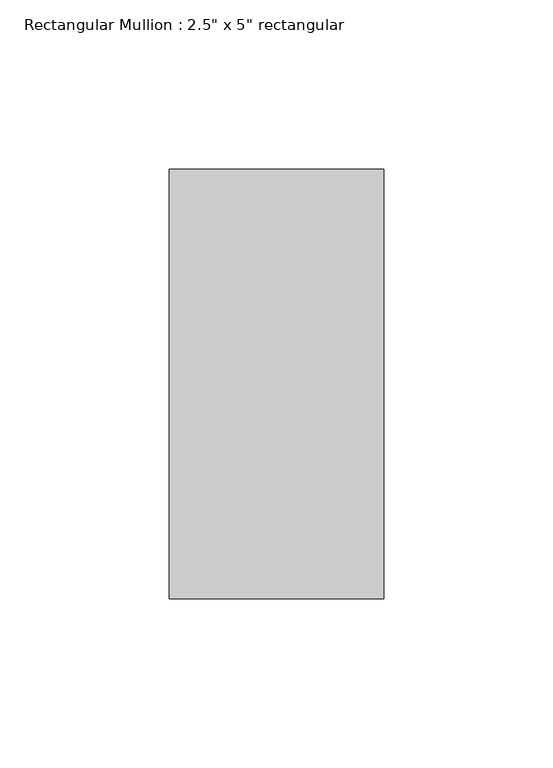
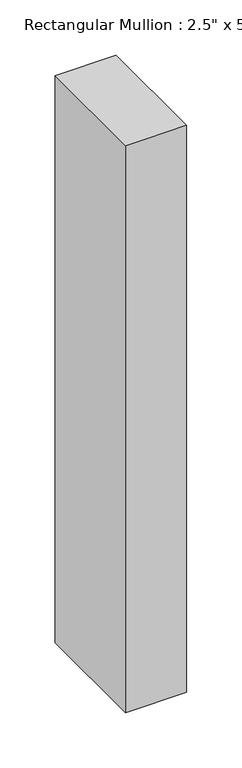
"""IFC4 building model written with IfcOpenShell, lengths in millimetres: member geometry."""

from ifc_helpers import new_model, si_unit, frame, origin, place, context, project, spatial, polyline, outline, extrude, source, transform, mapped, element, save


def member_2a256751(model_context):
    return source(origin(), model_context, "Body", "SweptSolid", [
        extrude(outline(polyline([(31.75, 63.5), (31.75, -63.5), (-31.75, -63.5), (-31.75, 63.5), (31.75, 63.5)])), frame((0.0, 0.0, -623.7034682), z_axis=(0.0, 0.0, 1.0), x_axis=(1.0, 0.0, 0.0)), (0.0, 0.0, 1.0), 623.7034682),
    ])


if __name__ == "__main__":
    model = new_model("IFC4")
    model_context = context("Model", 3, world=origin())
    ifc_project = project(units=[si_unit("LENGTHUNIT", "METRE", prefix="MILLI")], contexts=[model_context])
    site = spatial("IfcSite", under=ifc_project)
    building = spatial("IfcBuilding", under=site)
    placement = place(None, origin())
    member_shape = member_2a256751(model_context)
    element("IfcMember", 1, ObjectType="Rectangular Mullion : 2.5\" x 5\" rectangular", at=placement, inside=building, context=model_context, shape_type="MappedRepresentation", body=[
        mapped(member_shape, transform((0.0, 0.0, 0.0), x_axis=(1.0, 0.0, 0.0), y_axis=(0.0, 1.0, 0.0), z_axis=(0.0, 0.0, 1.0))),
    ])
    save(model, "model.ifc")

# Revit data of these elements
# Type "Rectangular Mullion : 2.5\" x 5\" rectangular"
#   built-in parameter 1007304 = 0.416667 (stored number, unit not read)
#   built-in parameter 1007301 = 0.104167 (stored number, unit not read)
#   built-in parameter 1007300 = 0.104167 (stored number, unit not read)
# Element 1 (IfcMember, "Rectangular Mullion : 2.5\" x 5\" rectangular")
#   Materials on its faces: "BLACK COLOUR"
# Materials
#   "BLACK COLOUR": class "Generic", colour RGB 120 120 120, transparency 0, Cost = 0
